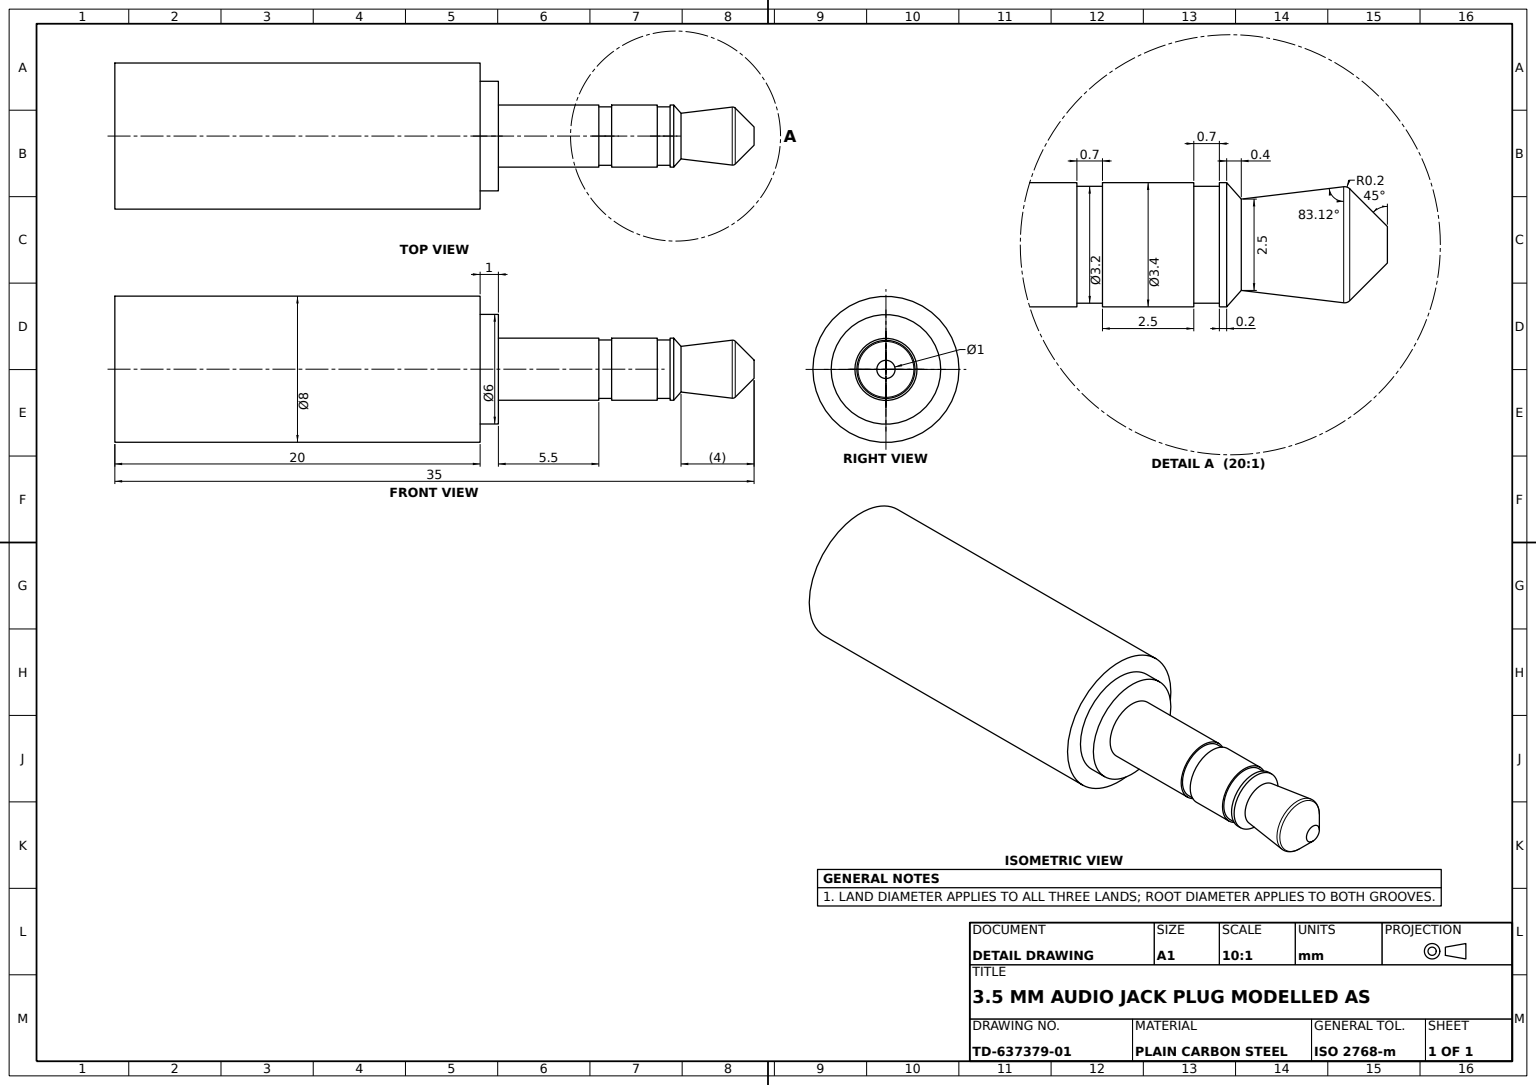
SolidWorks part; units mm, degrees
material "Plain Carbon Steel"
ref_plane "Front Plane" through (0, 0, 0) normal (0, 0, 1) x (1, 0, 0)
ref_plane "Top Plane" through (0, 0, 0) normal (0, 1, 0) x (1, 0, 0)
ref_plane "Right Plane" through (0, 0, 0) normal (1, 0, 0) x (0, 0, -1)
sketch "Plug Profile Sketch" plane through (0, 0, 0) normal (0, 0, 1) x (1, 0, 0)
  line L0 (0, 0) -> (-35, 0)
  line L1 (-35, 0) -> (-35, 4)
  line L2 (-35, 4) -> (-15, 4)
  line L3 (-15, 4) -> (-15, 3)
  line L4 (-15, 3) -> (-14, 3)
  line L5 (-14, 3) -> (-14, 1.7)
  line L6 (-14, 1.7) -> (-8.5, 1.7)
  line L7 (-8.5, 1.7) -> (-8.5, 1.6)
  line L8 (-8.5, 1.6) -> (-7.8, 1.6)
  line L9 (-7.8, 1.6) -> (-7.8, 1.7)
  line L10 (-7.8, 1.7) -> (-5.3, 1.7)
  line L11 (-5.3, 1.7) -> (-5.3, 1.6)
  line L12 (-5.3, 1.6) -> (-4.6, 1.6)
  line L13 (-4.6, 1.6) -> (-4.6, 1.7)
  line L14 (-4.6, 1.7) -> (-4.4, 1.7)
  line L15 (-4.4, 1.7) -> (-4, 1.25)
  line L16 (-4, 1.25) -> (-1.1, 1.6)
  line L17 (-1.1, 1.6) -> (0, 0.5)
  line L18 (0, 0.5) -> (0, 0)
  dimension "D1" = 35
  dimension "D2" = 4
  dimension "D3" = 3
  dimension "D4" = 1
  dimension "D5" = 1.7
  dimension "D6" = 5.5
  dimension "D7" = 0.7
  dimension "D8" = 0.7
  dimension "D9" = 2.5
  dimension "D10" = 0.1
  dimension "D11" = 0.2
  dimension "D12" = 1.25
  dimension "D13" = 0.4
  dimension "D14" = 1.6
  dimension "D15" = 0.5
  dimension "D16" = 135
  dimension "D17" = 20
revolve "Plug Body Revolve" add sketch "Plug Profile Sketch" angle 360 about L0
fillet "Edge Fillet R0.2" radius 0.2 1 edges at (-1.1, 0, -1.6)
